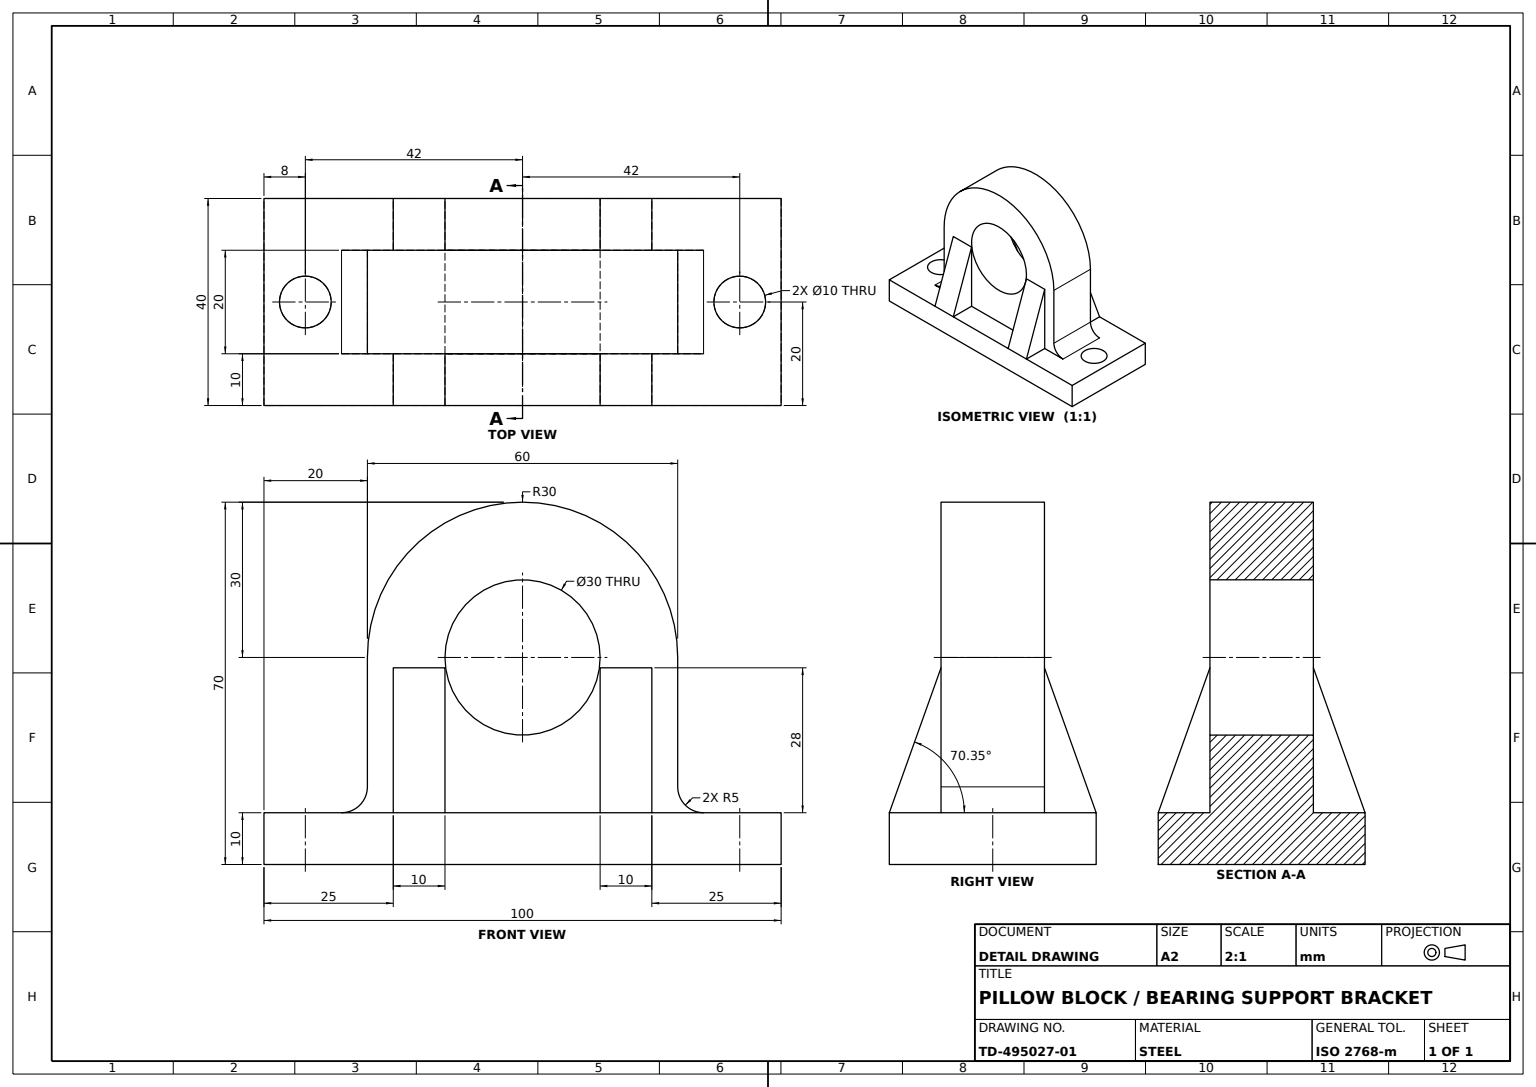
from build123d import *

# Parameters (mm, degrees)
BASE_PLATE_DEPTH                    = 20
SKETCH1_4_R                         = 15
BEARING_HOUSING_DEPTH               = 10
HOUSING_FILLET_R5_A_R               = 5
HOUSING_FILLET_R5_B_R               = 5
SUPPORT_START                       = 25
SUPPORT_RIB_DEPTH                   = 10
RIB_START                           = 25
RIB_MIRROR_FRONT_PLANE_COPY_1_DEPTH = 10
MOUNTING_HOLE_SKETCH_R              = 5
MOUNTING_HOLE_10_DEPTH              = 89.317608663


with BuildPart() as part:
    # Bracket Profile Sketch → Base Plate (new, symmetric)
    with BuildSketch(Plane.XY):
        Polygon((-50, 0), (0, 0), (0, 10), (-30, 10), (-50, 10), align=None)
        Polygon((0, 10), (0, 0), (50, 0), (50, 10), (30, 10), align=None)
    extrude(amount=BASE_PLATE_DEPTH, both=True)

    # Sketch1_4 → Bearing Housing (add, symmetric)
    # profile 1 of 2: a face of its own
    with BuildSketch(Plane.XY):
        Polygon((-50, 10), (-50, 0), (50, 0), (50, 10), (30, 10), (-30, 10), align=None)
    # profile 2 of 2: a face of its own
    with BuildSketch(Plane.XY):
        with BuildLine():
            Line((-30, 40), (-30, 10))
            Line((-30, 10), (30, 10))
            Line((30, 10), (30, 40))
            ThreePointArc((30, 40), (0, 70), (-30, 40))
        make_face()
        with Locations((0, 40)):
            Circle(SKETCH1_4_R, mode=Mode.SUBTRACT)
    extrude(amount=BEARING_HOUSING_DEPTH, both=True)

    # Housing Fillet R5 A
    housing_fillet_r5_a_edges = [part.edges().sort_by_distance(p)[0] for p in [
        (30, 10, 0),
    ]]
    fillet(housing_fillet_r5_a_edges, radius=HOUSING_FILLET_R5_A_R)

    # Housing Fillet R5 B
    housing_fillet_r5_b_edges = [part.edges().sort_by_distance(p)[0] for p in [
        (-30, 10, 0),
    ]]
    fillet(housing_fillet_r5_b_edges, radius=HOUSING_FILLET_R5_B_R)

    # Support Rib Sketch → Support Rib (add)
    with BuildSketch(Plane(origin=(0, 0, 0), x_dir=(0, 0, -1), z_dir=(1, 0, 0)).offset(SUPPORT_START)):
        Polygon((20, 10), (10, 38), (10, 10), align=None)
    support_rib = extrude(amount=-SUPPORT_RIB_DEPTH)

    # Rib Mirror Right Plane: Support Rib across plane
    add(support_rib.mirror(Plane(origin=(0, 0, 0), x_dir=(0, 0, 1), z_dir=(1, 0, 0))))

    # Rib Mirror Front Plane: Support Rib across plane
    add(support_rib.mirror(Plane.XY))

    # Rib Mirror Front Plane copy 1 sketch → Rib Mirror Front Plane copy 1 (add)
    with BuildSketch(Plane.ZY.offset(RIB_START)):
        Polygon((20, 10), (10, 38), (10, 10), align=None)
    extrude(amount=-RIB_MIRROR_FRONT_PLANE_COPY_1_DEPTH)

    # Mounting Hole Sketch → Mounting Hole _10 (cut, through all)
    with BuildSketch(Plane(origin=(0, 0, 0), x_dir=(1, 0, 0), z_dir=(0, 1, 0))):
        with Locations(Location((-42, 0, 0), (0, 0, 270))):
            Circle(MOUNTING_HOLE_SKETCH_R)
    mounting_hole_10 = extrude(amount=MOUNTING_HOLE_10_DEPTH, mode=Mode.SUBTRACT)

    # Mounting Hole Mirror: Mounting Hole _10 across plane
    add(mounting_hole_10.mirror(Plane(origin=(0, 0, 0), x_dir=(0, 0, 1), z_dir=(1, 0, 0))), mode=Mode.SUBTRACT)


solid = part.part
